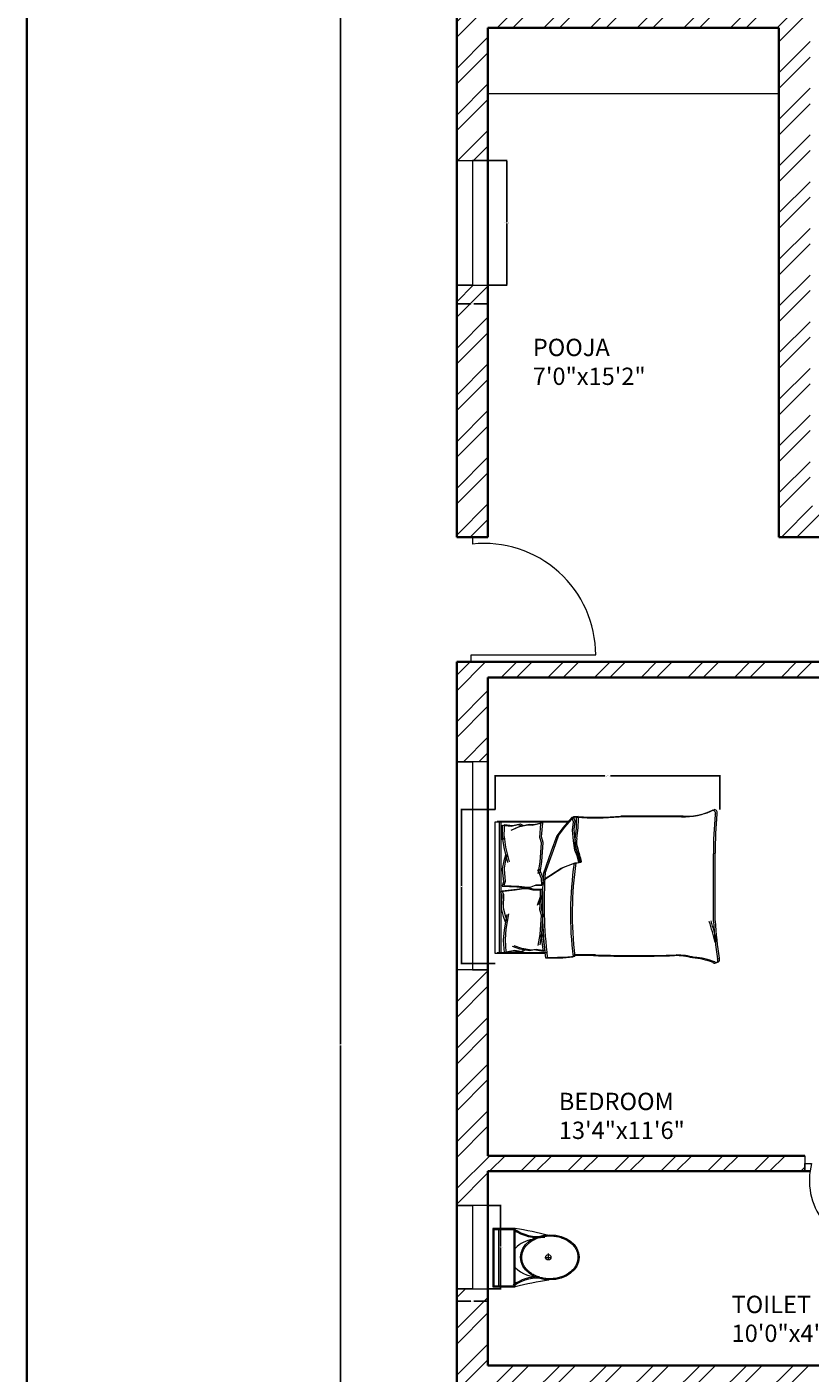
# Model space of a CAD drawing. Units: inches. Extents: x 1152 to 2588, y 1459 to 2618.
# Tile 4 of 17: x 1152 to 1378, y 1843 to 2231. Entities that reach past the tile are written whole.
import ezdxf

# ---------------------------------------------------------------- set-up
doc = ezdxf.new("R2010")
doc.units = ezdxf.units.IN
for name, color, linetype, lineweight in [('A-ANNO-DIMS', 2, 'Continuous', 18), ('A-ANNO-TTLB', 7, 'Continuous', 35), ('A-AREA-IDEN', 7, 'Continuous', 18), ('A-DOOR', 4, 'Continuous', 18), ('A-FLOR-CASE', 30, 'Continuous', 18), ('A-FLOR-FIXT', 9, 'Continuous', 18), ('A-FURN', 8, 'Continuous', 13), ('A-GLAZ', 4, 'Continuous', 18), ('A-WALL', 7, 'Continuous', 35), ('A-WALL-PATT', 8, 'Continuous', 13)]:
    doc.layers.add(name, color=color, linetype=linetype, lineweight=lineweight)
doc.styles.get("Standard").update_dxf_attribs({"font": 'arial.ttf'})
doc.dimstyles.get("Standard").update_dxf_attribs({"dimtxt": 0.18, "dimasz": 0.18, "dimexe": 0.18, "dimexo": 0.0625, "dimgap": 0.09, "dimtad": 0, "dimtih": 1, "dimtoh": 1, "dimdec": 4, "dimzin": 0, "dimdsep": 46, "dimtxsty": 'Standard', "dimcen": 0.09, "dimadec": 0, "dimazin": 0, "dimtfac": 1, "dimtdec": 4, "dimtofl": 0, "dimtmove": 0, "dimatfit": 3, "dimfxl": 1, "dimtolj": 1, "dimtzin": 0, "dimarcsym": 0})

# ---------------------------------------------------------------- blocks, each defined once
blk = doc.blocks.new('A$C31115884')
for p, q in [((283, 498), (223, 498)), ((258, 466), (258, 523)), ((0, 200), (0, 0)), ((520, 200), (0, 200)), ((10, 190), (10, 10)), ((510, 190), (10, 190)), ((510, 10), (510, 190)), ((520, 0), (520, 200)), ((510, 54), (0, 54)), ((10, 10), (510, 10)), ((0, 0), (520, 0))]:
    blk.add_line(p, q)
blk.add_circle((256, 496), 23.6)
for centre, radius, start, end in [((2778, -205), 2807, 165.4549, 171.7133), ((3237, 905), 2807, 188.2867, 194.5451), ((-295, 403), 365, 324.2091, 9.3499), ((-295, 403), 375, 324.2091, 9.3499), ((139, 406), 293, 315.8436, 2.6563), ((806, 403), 375, 179.2036, 215.7909), ((806, 403), 365, 170.6501, 215.7909), ((384, 406), 293, 190.2774, 224.1564)]:
    blk.add_arc(centre, radius, start, end)
blk.add_ellipse((256, 510), major_axis=(0, -261), ratio=0.772727)
blk.add_open_spline([(256, 259), (263, 259), (270, 260), (288, 262), (299, 265), (320, 273), (330, 278), (350, 291), (360, 299), (378, 316), (386, 326), (402, 347), (409, 358), (421, 383), (427, 395), (436, 422), (440, 436), (445, 465), (447, 480), (448, 509), (448, 524), (445, 553), (443, 568), (436, 596), (432, 610), (422, 636), (416, 649), (402, 672), (395, 683), (379, 703), (370, 712), (351, 728), (341, 735), (321, 746), (310, 751), (289, 757), (278, 759), (256, 761), (245, 761), (223, 757), (212, 754), (191, 746), (181, 741), (161, 728), (151, 720), (133, 703), (125, 693), (110, 672), (103, 660), (90, 636), (85, 623), (76, 596), (72, 582), (67, 553), (66, 538), (64, 509), (65, 494), (68, 465), (70, 450), (77, 422), (81, 408), (91, 382), (97, 370), (111, 346), (118, 335), (135, 316), (144, 307), (162, 291), (172, 284), (193, 273), (203, 269), (225, 262), (236, 260), (250, 259), (253, 259), (256, 259)], degree=3, knots=[0, 0, 0, 0, 0.110105, 0.110105, 0.285049, 0.285049, 0.459994, 0.459994, 0.634938, 0.634938, 0.809882, 0.809882, 0.984827, 0.984827, 1.159771, 1.159771, 1.334715, 1.334715, 1.50966, 1.50966, 1.684604, 1.684604, 1.859549, 1.859549, 2.034493, 2.034493, 2.209437, 2.209437, 2.384382, 2.384382, 2.559326, 2.559326, 2.73427, 2.73427, 2.909215, 2.909215, 3.084159, 3.084159, 3.259103, 3.259103, 3.434048, 3.434048, 3.608992, 3.608992, 3.783936, 3.783936, 3.958881, 3.958881, 4.133825, 4.133825, 4.30877, 4.30877, 4.483714, 4.483714, 4.658658, 4.658658, 4.833603, 4.833603, 5.008547, 5.008547, 5.183491, 5.183491, 5.358436, 5.358436, 5.53338, 5.53338, 5.708324, 5.708324, 5.883269, 5.883269, 6.058213, 6.058213, 6.233158, 6.233158, 6.283185, 6.283185, 6.283185, 6.283185])
blk = doc.blocks.new('BED-PLAN')
for p, q in [((49.83, 41.36), (64.23, 41.36)), ((49.83, 41.36), (64.23, 41.36)), ((50.34, 41.54), (64.74, 41.54)), ((50.34, 41.54), (64.74, 41.54)), ((51.02, 36.75), (50.45, 40.8)), ((50.45, 40.8), (52.97, 40.34)), ((51.02, 36.75), (50.45, 40.8)), ((50.45, 40.8), (52.97, 40.34)), ((51.53, 36.93), (50.95, 40.98)), ((50.95, 40.98), (53.48, 40.52)), ((51.53, 36.93), (50.95, 40.98)), ((50.95, 40.98), (53.48, 40.52)), ((51.81, 39.05), (51.28, 35.85)), ((51.81, 39.05), (51.28, 35.85)), ((52.32, 39.23), (51.79, 36.03)), ((52.32, 39.23), (51.79, 36.03)), ((52.97, 40.34), (54.24, 40.57)), ((52.97, 40.34), (54.24, 40.57)), ((53.48, 40.52), (54.75, 40.75)), ((53.48, 40.52), (54.75, 40.75)), ((54.24, 40.57), (57.11, 40.11)), ((54.24, 40.57), (57.11, 40.11)), ((54.75, 40.75), (57.62, 40.29)), ((54.75, 40.75), (57.62, 40.29)), ((57, 40.91), (56.19, 40.45)), ((57, 40.91), (56.19, 40.45)), ((57.51, 41.09), (56.7, 40.64)), ((57.51, 41.09), (56.7, 40.64)), ((59.07, 40.57), (57, 40.91)), ((59.07, 40.57), (57, 40.91)), ((57.11, 40.11), (59.3, 39.3)), ((57.11, 40.11), (59.3, 39.3)), ((59.57, 40.75), (57.51, 41.09)), ((59.57, 40.75), (57.51, 41.09)), ((57.62, 40.29), (59.8, 39.49)), ((57.62, 40.29), (59.8, 39.49)), ((61.59, 41.03), (59.07, 40.57)), ((61.59, 41.03), (59.07, 40.57)), ((62.1, 41.21), (59.57, 40.75)), ((62.1, 41.21), (59.57, 40.75)), ((61.58, 41.03), (61.84, 37.62)), ((61.58, 41.02), (61.84, 37.62)), ((62.08, 41.21), (62.35, 37.8)), ((62.08, 41.21), (62.35, 37.8)), ((63.01, 41.36), (63.01, 3.37)), ((63.01, 41.36), (63.01, 3.37)), ((63.52, 41.54), (63.52, 3.56)), ((63.52, 41.54), (63.52, 3.56)), ((64.74, 41.54), (64.74, 3.56)), ((51.28, 35.85), (50.93, 30.27)), ((51.28, 35.85), (50.93, 30.27)), ((51.28, 35.85), (51.02, 36.75)), ((51.28, 35.85), (51.02, 36.75)), ((51.79, 36.03), (51.44, 30.46)), ((51.79, 36.03), (51.44, 30.46)), ((51.79, 36.03), (51.53, 36.93)), ((51.79, 36.03), (51.53, 36.93)), ((61.82, 37.54), (61.59, 34.5)), ((61.82, 37.54), (61.59, 34.5)), ((61.84, 37.62), (61.82, 37.54)), ((61.84, 37.62), (61.82, 37.54)), ((62.33, 37.72), (62.1, 34.68)), ((62.33, 37.72), (62.1, 34.68)), ((62.35, 37.8), (62.33, 37.72)), ((62.35, 37.8), (62.33, 37.72)), ((1.24, 32.15), (1.24, 12.59)), ((1.24, 32.15), (1.24, 12.59)), ((1.75, 32.33), (1.75, 12.77)), ((1.75, 32.33), (1.75, 12.77)), ((61.59, 34.5), (60.79, 30.13)), ((61.59, 34.5), (60.79, 30.13)), ((61.25, 32.32), (61.82, 30.71)), ((61.25, 32.32), (61.82, 30.71)), ((62.1, 34.68), (61.3, 30.31)), ((62.1, 34.68), (61.3, 30.31)), ((61.76, 32.5), (62.33, 30.89)), ((61.76, 32.5), (62.33, 30.89)), ((50.93, 30.27), (51.38, 28.72)), ((50.93, 30.27), (51.38, 28.72)), ((51.38, 28.72), (51.06, 24.64)), ((51.38, 28.72), (51.06, 24.64)), ((51.3, 24.96), (52.17, 27.46)), ((51.3, 24.96), (52.17, 27.46)), ((51.44, 30.46), (51.89, 28.9)), ((51.44, 30.46), (51.89, 28.9)), ((51.89, 28.9), (51.56, 24.82)), ((51.89, 28.9), (51.56, 24.82)), ((51.81, 25.15), (52.68, 27.65)), ((51.81, 25.15), (52.68, 27.65)), ((61.82, 30.71), (62.4, 28.41)), ((61.82, 30.71), (62.4, 28.41)), ((62.4, 28.15), (62.28, 24.62)), ((62.4, 28.15), (62.28, 24.62)), ((62.33, 30.89), (62.91, 28.59)), ((62.33, 30.89), (62.91, 28.59)), ((62.4, 28.41), (62.4, 28.15)), ((62.4, 28.41), (62.4, 28.15)), ((62.91, 28.34), (62.79, 24.8)), ((62.91, 28.34), (62.79, 24.8)), ((62.91, 28.59), (62.91, 28.34)), ((62.91, 28.59), (62.91, 28.34)), ((51.3, 23.01), (51.3, 24.96)), ((51.3, 23.01), (51.3, 24.96)), ((51.81, 23.19), (51.81, 25.15)), ((51.81, 23.19), (51.81, 25.15)), ((62.74, 23.47), (58.49, 23.01)), ((62.74, 23.47), (58.49, 23.01)), ((63.25, 23.65), (59, 23.19)), ((63.25, 23.65), (59, 23.19)), ((62.28, 24.62), (62.74, 23.47)), ((62.28, 24.62), (62.74, 23.47)), ((62.79, 24.8), (63.25, 23.65)), ((62.79, 24.8), (63.25, 23.65)), ((50.41, 20.07), (45.25, 16.74)), ((50.41, 20.07), (45.25, 16.74)), ((50.92, 20.25), (45.76, 16.92)), ((50.92, 20.25), (45.76, 16.92)), ((52.93, 21.76), (50.8, 21.63)), ((52.93, 21.76), (50.8, 21.63)), ((50.8, 21.63), (50.92, 19.68)), ((50.8, 21.63), (50.92, 19.68)), ((50.92, 19.68), (51.95, 17.24)), ((50.92, 19.68), (51.95, 17.24)), ((53.43, 23.01), (51.3, 23.01)), ((53.43, 23.01), (51.3, 23.01)), ((53.44, 21.95), (51.31, 21.81)), ((53.44, 21.94), (51.31, 21.81)), ((51.31, 21.81), (51.43, 19.86)), ((51.31, 21.81), (51.43, 19.86)), ((51.43, 19.86), (52.45, 17.42)), ((51.43, 19.86), (52.45, 17.42)), ((53.94, 23.19), (51.81, 23.19)), ((53.94, 23.19), (51.81, 23.19)), ((54.39, 22.32), (52.93, 21.76)), ((54.39, 22.32), (52.93, 21.76)), ((54.93, 22.55), (53.43, 23.01)), ((54.93, 22.55), (53.43, 23.01)), ((54.9, 22.5), (53.44, 21.94)), ((54.9, 22.5), (53.44, 21.95)), ((55.44, 22.73), (53.94, 23.19)), ((55.44, 22.73), (53.94, 23.19)), ((55.42, 22.38), (54.39, 22.32)), ((55.42, 22.38), (54.39, 22.32)), ((55.93, 22.56), (54.9, 22.5)), ((55.93, 22.56), (54.9, 22.5)), ((55.96, 22.55), (54.93, 22.55)), ((55.96, 22.55), (54.93, 22.55)), ((57.98, 22.08), (55.42, 22.38)), ((57.98, 22.08), (55.42, 22.38)), ((56.47, 22.73), (55.44, 22.73)), ((56.47, 22.73), (55.44, 22.73)), ((58.48, 22.26), (55.93, 22.56)), ((58.48, 22.26), (55.93, 22.56)), ((58.49, 23.01), (55.96, 22.55)), ((58.49, 23.01), (55.96, 22.55)), ((59, 23.19), (56.47, 22.73)), ((59, 23.19), (56.47, 22.73)), ((62.25, 21.89), (57.98, 22.08)), ((62.25, 21.89), (57.98, 22.08)), ((62.76, 22.07), (58.48, 22.26)), ((62.76, 22.07), (58.48, 22.26)), ((61.86, 20.71), (62.25, 21.89)), ((61.86, 20.71), (62.25, 21.89)), ((62.2, 17.19), (61.86, 20.71)), ((62.2, 17.19), (61.86, 20.71)), ((62.37, 20.89), (62.76, 22.07)), ((62.37, 20.89), (62.76, 22.07)), ((62.71, 17.37), (62.37, 20.89)), ((62.71, 17.37), (62.37, 20.89)), ((42.19, 15.57), (40.59, 15.32)), ((42.19, 15.57), (40.59, 15.32)), ((45.25, 16.74), (41.68, 15.39)), ((45.25, 16.74), (41.68, 15.39)), ((45.76, 16.92), (42.19, 15.57)), ((45.76, 16.92), (42.19, 15.57)), ((48.08, 11.82), (50.41, 18.44)), ((48.08, 11.82), (50.41, 18.44)), ((48.59, 12), (50.92, 18.63)), ((48.59, 12), (50.92, 18.63)), ((51.81, 18.24), (51.28, 15.03)), ((51.81, 18.24), (51.28, 15.03)), ((52.32, 18.42), (51.79, 15.22)), ((52.32, 18.42), (51.79, 15.22)), ((61.78, 14.61), (62.21, 16.94)), ((61.78, 14.61), (62.21, 16.94)), ((62.21, 16.94), (62.2, 17.19)), ((62.21, 16.94), (62.2, 17.19)), ((62.29, 14.79), (62.72, 17.12)), ((62.29, 14.79), (62.72, 17.12)), ((62.72, 17.12), (62.71, 17.37)), ((62.72, 17.12), (62.71, 17.37)), ((41.68, 15.39), (40.08, 15.14)), ((41.68, 15.39), (40.08, 15.14)), ((40.08, 15.14), (40.58, 13.17)), ((40.08, 15.14), (40.58, 13.17)), ((40.58, 13.17), (41.31, 11.57)), ((40.58, 13.17), (41.31, 11.57)), ((40.59, 15.32), (41.08, 13.35)), ((40.59, 15.32), (41.08, 13.35)), ((41.08, 13.35), (41.82, 11.75)), ((41.08, 13.35), (41.82, 11.75)), ((41.82, 11.75), (42.19, 9.04)), ((41.82, 11.75), (42.19, 9.04)), ((46.48, 7.38), (48.08, 11.82)), ((46.48, 7.38), (48.08, 11.82)), ((46.99, 7.57), (48.59, 12)), ((46.99, 7.57), (48.59, 12)), ((51.28, 15.03), (50.93, 9.46)), ((51.28, 15.03), (50.93, 9.46)), ((51.79, 15.22), (51.44, 9.64)), ((51.79, 15.22), (51.44, 9.64)), ((61.79, 10.81), (60.71, 15.11)), ((61.79, 10.81), (60.71, 15.11)), ((62.3, 10.99), (61.22, 15.3)), ((62.3, 10.99), (61.22, 15.3)), ((61.31, 12.96), (61.78, 14.61)), ((61.31, 12.96), (61.78, 14.61)), ((61.82, 13.15), (62.29, 14.79)), ((61.82, 13.15), (62.29, 14.79)), ((41.31, 11.57), (41.68, 8.86)), ((41.31, 11.57), (41.68, 8.86)), ((41.68, 8.86), (41.93, 5.78)), ((41.68, 8.86), (41.93, 5.78)), ((42.19, 9.04), (42.44, 5.97)), ((42.19, 9.04), (42.44, 5.97)), ((50.93, 9.46), (51.38, 7.9)), ((50.93, 9.46), (51.38, 7.9)), ((51.38, 7.9), (51.06, 3.82)), ((51.38, 7.9), (51.06, 3.82)), ((51.44, 9.64), (51.89, 8.09)), ((51.44, 9.64), (51.89, 8.09)), ((51.89, 8.09), (51.56, 4.01)), ((51.89, 8.09), (51.56, 4.01)), ((62.21, 7.79), (61.79, 10.81)), ((62.21, 7.79), (61.79, 10.81)), ((62.2, 4.29), (62.27, 8.59)), ((62.2, 4.29), (62.27, 8.58)), ((62.27, 8.59), (62.21, 7.79)), ((62.27, 8.58), (62.21, 7.79)), ((62.72, 7.97), (62.3, 10.99)), ((62.72, 7.97), (62.3, 10.99)), ((62.71, 4.47), (62.78, 8.77)), ((62.71, 4.47), (62.78, 8.77)), ((62.78, 8.77), (62.72, 7.97)), ((62.78, 8.77), (62.72, 7.97)), ((41.93, 5.78), (41.68, 3.32)), ((41.93, 5.78), (41.68, 3.32)), ((42.18, 2.1), (44.76, 5.05)), ((42.18, 2.1), (44.76, 5.05)), ((42.44, 5.97), (42.19, 3.5)), ((42.44, 5.97), (42.19, 3.5)), ((42.68, 2.28), (45.27, 5.23)), ((42.68, 2.28), (45.27, 5.23)), ((44.76, 5.05), (46.48, 7.38)), ((44.76, 5.05), (46.48, 7.38)), ((45.27, 5.23), (46.99, 7.57)), ((45.27, 5.23), (46.99, 7.57)), ((51.06, 3.82), (53.55, 4.44)), ((51.06, 3.82), (53.55, 4.44)), ((51.56, 4.01), (54.06, 4.62)), ((51.56, 4.01), (54.06, 4.62)), ((53.55, 4.44), (54.83, 4.29)), ((53.55, 4.44), (54.83, 4.29)), ((54.06, 4.62), (55.34, 4.47)), ((54.06, 4.62), (55.34, 4.47)), ((54.83, 4.29), (57.67, 4.93)), ((54.83, 4.29), (57.67, 4.93)), ((55.34, 4.47), (58.17, 5.11)), ((55.34, 4.47), (58.17, 5.11)), ((57.6, 4.12), (56.77, 4.53)), ((57.6, 4.12), (56.77, 4.53)), ((58.11, 4.3), (57.28, 4.71)), ((58.11, 4.3), (57.28, 4.71)), ((59.65, 4.59), (57.6, 4.12)), ((59.65, 4.59), (57.6, 4.12)), ((57.67, 4.93), (59.8, 5.87)), ((57.67, 4.93), (59.8, 5.87)), ((60.15, 4.77), (58.11, 4.3)), ((60.15, 4.77), (58.11, 4.3)), ((58.17, 5.11), (60.3, 6.05)), ((58.17, 5.11), (60.3, 6.05)), ((62.2, 4.29), (59.65, 4.59)), ((62.2, 4.29), (59.65, 4.59)), ((62.71, 4.47), (60.15, 4.77)), ((62.71, 4.47), (60.15, 4.77)), ((40.79, 2.04), (42.18, 2.1, 3.08)), ((40.79, 2.04), (42.18, 2.1, 3.08)), ((41.3, 2.22), (42.68, 2.28, 3.08)), ((41.3, 2.22), (42.68, 2.28, 3.08)), ((41.68, 3.32), (42.18, 2.1)), ((41.68, 3.32), (42.18, 2.1)), ((42.19, 3.5), (42.68, 2.28)), ((42.19, 3.5), (42.68, 2.28)), ((64.23, 3.37), (43.08, 3.37)), ((64.23, 3.37), (43.08, 3.37)), ((64.74, 3.56), (43.59, 3.56)), ((64.74, 3.56), (43.59, 3.56))]:
    blk.add_line(p, q)
for centre, radius, start, end in [((0.86, 43.26), 0.866, 56.1736, 203.4781), ((0.86, 43.26), 0.866, 56.1736, 203.4781), ((-95.41, 27.09), 96.78, 2.9958, 9.4091), ((-95.41, 27.09), 96.78, 2.9958, 9.4091), ((1.37, 43.44), 0.866, 56.1736, 203.4781), ((1.37, 43.44), 0.866, 56.1736, 203.4781), ((-94.9, 27.27), 96.78, 2.9958, 9.4091), ((-94.9, 27.27), 96.78, 2.9958, 9.4091), ((8.37, 61.34), 18.73, 247.9751, 266.652), ((8.37, 61.34), 18.73, 247.9751, 266.652), ((8.88, 61.52), 18.73, 247.9751, 266.652), ((8.88, 61.52), 18.73, 247.9751, 266.652), ((13.46, 65.69), 23.56, 256.0648, 268.9113), ((13.46, 65.69), 23.56, 256.0648, 268.9113), ((48.76, -23.39), 66.22, 88.7218, 95.604), ((48.76, -23.39), 66.22, 88.7218, 95.604), ((-79.97, 27.33), 131.13, 356.0865, 6.7821), ((-79.97, 27.33), 131.13, 356.0865, 6.7821), ((12.95, 65.51), 23.56, 256.0648, 268.9113), ((12.95, 65.51), 23.56, 256.0648, 268.9113), ((24, -341.25), 383.38, 88.2277, 91.7185), ((24, -341.25), 383.38, 88.2277, 91.7185), ((24.51, -341.07), 383.38, 88.2277, 91.7185), ((24.51, -341.07), 383.38, 88.2277, 91.7185), ((39.45, 177.11), 135.22, 268.4762, 271.0082), ((39.45, 177.11), 135.22, 268.4762, 271.0082), ((39.96, 177.3), 135.22, 268.4762, 271.0082), ((39.96, 177.3), 135.22, 268.4762, 271.0082), ((-60.02, 30.01), 102.56, 351.7845, 6.9006), ((-60.02, 30.01), 102.56, 351.7845, 6.9006), ((48.26, -23.57), 66.22, 88.7218, 95.604), ((48.26, -23.57), 66.22, 88.7218, 95.604), ((-59.52, 30.19), 102.56, 351.7845, 6.9006), ((-59.52, 30.19), 102.56, 351.7845, 6.9006), ((-80.48, 27.15), 131.13, 356.0865, 6.7821), ((-80.48, 27.15), 131.13, 356.0865, 6.7821), ((83.08, 57.81), 84.62, 193.3832, 197.7053), ((83.08, 57.81), 84.62, 193.3832, 197.7053), ((83.59, 57.99), 84.62, 193.3832, 197.7053), ((83.59, 57.99), 84.62, 193.3832, 197.7053), ((-104.51, 11.41), 105.75, 354.4998, 0.6351), ((-104.51, 11.41), 105.75, 354.4998, 0.6351), ((-104, 11.59), 105.75, 354.4998, 0.6351), ((-104, 11.59), 105.75, 354.4998, 0.6351), ((40.03, 15), 0.147, 70.2464, 181.1377), ((40.03, 15), 0.147, 70.2464, 181.1377), ((63.05, 19.36), 23.57, 190.6617, 199.8806), ((63.05, 19.36), 23.57, 190.6617, 199.8806), ((40.54, 15.18), 0.147, 70.2464, 181.1377), ((40.54, 15.18), 0.147, 70.2464, 181.1377), ((63.56, 19.54), 23.57, 190.6617, 199.8806), ((63.56, 19.54), 23.57, 190.6617, 199.8806), ((69.52, 3.32), 28.76, 169.8763, 182.5657), ((69.52, 3.32), 28.76, 169.8763, 182.5657), ((36.36, 9.35), 4.95, 348.6608, 23.7384), ((36.36, 9.35), 4.95, 348.6608, 23.7384), ((70.03, 3.51), 28.76, 169.8763, 182.5657), ((70.03, 3.51), 28.76, 169.8763, 182.5657), ((36.86, 9.53), 4.95, 348.6608, 23.7384), ((36.86, 9.53), 4.95, 348.6608, 23.7384), ((1.54, 0.87), 0.876, 152.6588, 266.02), ((1.54, 0.87), 0.876, 152.6588, 266.02), ((2.05, 1.06), 0.876, 152.6588, 266.02), ((2.05, 1.06), 0.876, 152.6588, 266.02), ((9.65, -16.41), 18.33, 87.4714, 116.4681), ((9.65, -16.41), 18.33, 87.4714, 116.4681), ((10.16, -16.23), 18.33, 87.4714, 116.4681), ((10.16, -16.23), 18.33, 87.4714, 116.4681), ((10.32, 3628.06), 3626.16, 270.00217, 270.28689), ((10.32, 3628.06), 3626.16, 270.00217, 270.28689), ((10.83, 3628.24), 3626.16, 270.00217, 270.28689), ((10.83, 3628.24), 3626.16, 270.00217, 270.28689), ((35.36, -100.76), 102.94, 86.9791, 93.8365), ((35.36, -100.76), 102.94, 86.9791, 93.8365), ((35.87, -100.58), 102.94, 86.9791, 93.8365), ((35.87, -100.57), 102.94, 86.9791, 93.8365)]:
    blk.add_arc(centre, radius, start, end)
blk = doc.blocks.new('DOOR-24-BATH-WEST')
for p, q in [((0, 26.25), (0, 21.75)), ((0, 21.75), (0, 24)), ((0, 24), (2, 24)), ((22.43, 24), (20.43, 24)), ((20.43, 24), (20.43, 0)), ((22.43, 21.75), (22.43, 26.25)), ((22.43, 26.25), (22.43, 24))]:
    blk.add_line(p, q)
blk.add_arc((20.43, 19.08), 19.08, 165.0504, 270)
blk = doc.blocks.new('DOOR-36-POOJA')
for p, q in [((0.4, 36), (0.4, 34)), ((0, 0), (0, 2)), ((0, 2), (36, 2))]:
    blk.add_line(p, q)
blk.add_arc((3.82, 2), 32.18, 0, 96.1017)
blk = doc.blocks.new('WIN-60-EXT')
for p, q in [((0, 9), (0, 0)), ((60, 4.5), (60, 9)), ((60, 9), (60, 0)), ((0, 0), (0, 4.5)), ((0, 4.5), (60, 4.5))]:
    blk.add_line(p, q)
blk = doc.blocks.new('WIN-36')
for p, q in [((0, 36), (9, 36)), ((9, 36), (4.5, 36)), ((4.5, 36), (4.5, 0)), ((4.5, 0), (0, 0)), ((0, 0), (9, 0))]:
    blk.add_line(p, q)
blk = doc.blocks.new('WIN-24-BATH-WEST')
for p, q in [((9, 24), (0, 24)), ((0, 24), (4.5, 24)), ((4.5, 24), (4.5, 0)), ((4.5, 0), (0, 0)), ((0, 0), (9, 0))]:
    blk.add_line(p, q)
blk = doc.blocks.new('*D28')
at = {"layer": 'A-ANNO-DIMS', "color": 0, "lineweight": -2, "transparency": 16777216}
for p, q in [((1285.48, 2192.75), (1291, 2192.75)), ((1290.82, 2192.57), (1290.82, 2174.93)), ((1290.82, 2156.93), (1290.82, 2174.57)), ((1285.48, 2156.75), (1291, 2156.75))]:
    blk.add_line(p, q, dxfattribs=at)
at = {"layer": 'A-ANNO-DIMS', "color": 0, "transparency": 16777216}
for points in [[(1290.79, 2192.57), (1290.85, 2192.57), (1290.82, 2192.75)], [(1290.79, 2156.93), (1290.85, 2156.93), (1290.82, 2156.75)]]:
    blk.add_solid(points, dxfattribs=at)
at = {"layer": 'Defpoints', "color": 0, "transparency": 16777216}
for p in [(1285.42, 2192.75), (1290.82, 2192.75), (1285.42, 2156.75)]:
    blk.add_point(p, dxfattribs=at)
at = {"layer": 'A-ANNO-DIMS', "color": 0, "transparency": 16777216, "insert": (1290.82, 2174.75), "char_height": 0.18, "attachment_point": 5}
blk.add_mtext('\\A1;WIN. 36 TYP.', dxfattribs=at)
blk = doc.blocks.new('*D29')
at = {"layer": 'A-ANNO-DIMS', "color": 0, "lineweight": -2, "transparency": 16777216}
for p, q in [((1276.42, 2156.69), (1276.42, 2151.17)), ((1285.42, 2156.69), (1285.42, 2151.17)), ((1276.6, 2151.35), (1280.46, 2151.35)), ((1285.24, 2151.35), (1281.37, 2151.35))]:
    blk.add_line(p, q, dxfattribs=at)
at = {"layer": 'A-ANNO-DIMS', "color": 0, "transparency": 16777216}
for points in [[(1276.6, 2151.38), (1276.6, 2151.32), (1276.42, 2151.35)], [(1285.24, 2151.38), (1285.24, 2151.32), (1285.42, 2151.35)]]:
    blk.add_solid(points, dxfattribs=at)
at = {"layer": 'Defpoints', "color": 0, "transparency": 16777216}
for p in [(1276.42, 2156.75), (1285.42, 2156.75), (1285.42, 2151.35)]:
    blk.add_point(p, dxfattribs=at)
at = {"layer": 'A-ANNO-DIMS', "color": 0, "transparency": 16777216, "insert": (1280.92, 2151.35), "char_height": 0.18, "attachment_point": 5}
blk.add_mtext('\\A1;9 TYP.', dxfattribs=at)
blk = doc.blocks.new('*D32')
at = {"layer": 'A-ANNO-DIMS', "color": 0, "lineweight": -2, "transparency": 16777216}
for p, q in [((1287.53, 2005.5), (1287.53, 2015.34)), ((1287.71, 2015.16), (1319.13, 2015.16)), ((1352.17, 2015.16), (1320.76, 2015.16)), ((1352.35, 2005.5), (1352.35, 2015.34))]:
    blk.add_line(p, q, dxfattribs=at)
at = {"layer": 'A-ANNO-DIMS', "color": 0, "transparency": 16777216}
for points in [[(1287.71, 2015.19), (1287.71, 2015.13), (1287.53, 2015.16)], [(1352.17, 2015.19), (1352.17, 2015.13), (1352.35, 2015.16)]]:
    blk.add_solid(points, dxfattribs=at)
at = {"layer": 'Defpoints', "color": 0, "transparency": 16777216}
for p in [(1287.53, 2015.16), (1287.53, 2005.43), (1352.35, 2005.43)]:
    blk.add_point(p, dxfattribs=at)
at = {"layer": 'A-ANNO-DIMS', "color": 0, "transparency": 16777216, "insert": (1319.94, 2015.16), "char_height": 0.18, "attachment_point": 5}
blk.add_mtext('\\A1;BED 65 TYP.', dxfattribs=at)
blk = doc.blocks.new('*D33')
at = {"layer": 'A-ANNO-DIMS', "color": 0, "lineweight": -2, "transparency": 16777216}
for p, q in [((1287.47, 2005.43), (1277.63, 2005.43)), ((1277.81, 2005.25), (1277.81, 1983.43)), ((1277.81, 1961.24), (1277.81, 1983.07)), ((1287.47, 1961.06), (1277.63, 1961.06))]:
    blk.add_line(p, q, dxfattribs=at)
at = {"layer": 'A-ANNO-DIMS', "color": 0, "transparency": 16777216}
for points in [[(1277.78, 2005.25), (1277.84, 2005.25), (1277.81, 2005.43)], [(1277.78, 1961.24), (1277.84, 1961.24), (1277.81, 1961.06)]]:
    blk.add_solid(points, dxfattribs=at)
at = {"layer": 'Defpoints', "color": 0, "transparency": 16777216}
for p in [(1287.53, 2005.43), (1277.81, 1961.06), (1287.53, 1961.06)]:
    blk.add_point(p, dxfattribs=at)
at = {"layer": 'A-ANNO-DIMS', "color": 0, "transparency": 16777216, "insert": (1277.81, 1983.25), "char_height": 0.18, "attachment_point": 5}
blk.add_mtext('\\A1;44 TYP.', dxfattribs=at)
blk = doc.blocks.new('*D56')
at = {"layer": 'A-ANNO-DIMS', "color": 0, "lineweight": -2, "transparency": 16777216}
for p, q in [((1285.48, 1891.13), (1289.2, 1891.13)), ((1289.02, 1890.95), (1289.02, 1879.31)), ((1289.02, 1867.31), (1289.02, 1878.95)), ((1285.48, 1867.13), (1289.2, 1867.13))]:
    blk.add_line(p, q, dxfattribs=at)
at = {"layer": 'A-ANNO-DIMS', "color": 0, "transparency": 16777216}
for points in [[(1288.99, 1890.95), (1289.05, 1890.95), (1289.02, 1891.13)], [(1288.99, 1867.31), (1289.05, 1867.31), (1289.02, 1867.13)]]:
    blk.add_solid(points, dxfattribs=at)
at = {"layer": 'Defpoints', "color": 0, "transparency": 16777216}
for p in [(1285.42, 1891.13), (1289.02, 1891.13), (1285.42, 1867.13)]:
    blk.add_point(p, dxfattribs=at)
at = {"layer": 'A-ANNO-DIMS', "color": 0, "transparency": 16777216, "insert": (1289.02, 1879.13), "char_height": 0.18, "attachment_point": 5}
blk.add_mtext('\\A1;WIN. 24 TYP.', dxfattribs=at)
blk = doc.blocks.new('*D57')
at = {"layer": 'A-ANNO-DIMS', "color": 0, "lineweight": -2, "transparency": 16777216}
for p, q in [((1276.42, 1867.07), (1276.42, 1863.35)), ((1285.42, 1867.07), (1285.42, 1863.35)), ((1276.6, 1863.53), (1280.46, 1863.53)), ((1285.24, 1863.53), (1281.37, 1863.53))]:
    blk.add_line(p, q, dxfattribs=at)
at = {"layer": 'A-ANNO-DIMS', "color": 0, "transparency": 16777216}
for points in [[(1276.6, 1863.56), (1276.6, 1863.5), (1276.42, 1863.53)], [(1285.24, 1863.56), (1285.24, 1863.5), (1285.42, 1863.53)]]:
    blk.add_solid(points, dxfattribs=at)
at = {"layer": 'Defpoints', "color": 0, "transparency": 16777216}
for p in [(1276.42, 1867.13), (1285.42, 1867.13), (1285.42, 1863.53)]:
    blk.add_point(p, dxfattribs=at)
at = {"layer": 'A-ANNO-DIMS', "color": 0, "transparency": 16777216, "insert": (1280.92, 1863.53), "char_height": 0.18, "attachment_point": 5}
blk.add_mtext('\\A1;9 TYP.', dxfattribs=at)
blk = doc.blocks.new('*D71')
at = {"layer": 'A-ANNO-DIMS', "color": 0, "lineweight": -2, "transparency": 16777216}
for p, q in [((1276.35, 2240.05), (1242.64, 2240.05)), ((1242.82, 2239.87), (1242.82, 1937.73)), ((1242.82, 1635.23), (1242.82, 1937.36)), ((1276.35, 1635.05), (1242.64, 1635.05))]:
    blk.add_line(p, q, dxfattribs=at)
at = {"layer": 'A-ANNO-DIMS', "color": 0, "transparency": 16777216}
for points in [[(1242.79, 2239.87), (1242.85, 2239.87), (1242.82, 2240.05)], [(1242.79, 1635.23), (1242.85, 1635.23), (1242.82, 1635.05)]]:
    blk.add_solid(points, dxfattribs=at)
at = {"layer": 'Defpoints', "color": 0, "transparency": 16777216}
for p in [(1242.82, 2240.05), (1276.42, 2240.05), (1276.42, 1635.05)]:
    blk.add_point(p, dxfattribs=at)
at = {"layer": 'A-ANNO-DIMS', "color": 0, "transparency": 16777216, "insert": (1242.82, 1937.55), "char_height": 0.18, "attachment_point": 5}
blk.add_mtext('\\A1;605', dxfattribs=at)

msp = doc.modelspace()

# ---------------------------------------------------------------- hatches: boundary and pattern name
at = {"layer": 'A-WALL-PATT'}
h = msp.add_hatch(dxfattribs=at)
h.set_pattern_fill('ANSI32', color=256)
h.paths.add_polyline_path([(1408.9272, 2240.0458), (1276.4165, 2240.0458), (1276.4165, 2192.7491), (1285.4165, 2192.7491), (1285.4165, 2231.0458), (1369.4165, 2231.0458), (1369.4165, 2084.0458), (1526.9165, 2084.0458), (1526.9165, 2096.3728), (1524.6665, 2096.3728), (1522.4165, 2096.3728), (1522.4165, 2093.0458), (1378.4165, 2093.0458), (1378.4165, 2231.0458), (1408.9272, 2231.0458)])
h.paths.add_polyline_path([(1736.4165, 2240.0458), (1468.9272, 2240.0458), (1468.9272, 2231.0458), (1522.4165, 2231.0458), (1522.4165, 2127.3313), (1526.9165, 2127.3313), (1526.9165, 2231.0458), (1574.9165, 2231.0458), (1574.9165, 2188.0458), (1579.4165, 2188.0458), (1579.4165, 2231.0458), (1727.4165, 2231.0458), (1727.4165, 2183.9728), (1736.4165, 2183.9728)])
h.paths.add_polyline_path([(1285.4165, 2156.7491), (1276.4165, 2156.7491), (1276.4165, 2084.0458), (1285.4165, 2084.0458)], flags=17)
h.paths.add_polyline_path([(1285.4165, 2043.5458), (1445.4165, 2043.5458), (1445.4165, 1943.6503), (1454.4165, 1943.6503), (1454.4165, 2048.0458), (1276.4165, 2048.0458), (1276.4165, 2019.2077), (1280.9165, 2019.2077), (1285.4165, 2019.2077)])
h.paths.add_polyline_path([(1285.4165, 1959.2077), (1276.4165, 1959.2077), (1276.4165, 1891.1319), (1280.9165, 1891.1319), (1285.4165, 1891.1319), (1285.4165, 1901.0458), (1376.8505, 1901.0458), (1376.8505, 1903.2958), (1376.8505, 1905.5458), (1285.4165, 1905.5458)])
h.paths.add_polyline_path([(1518.4165, 1905.5458), (1399.2832, 1905.5458), (1399.2832, 1903.2958), (1399.2832, 1901.0458), (1405.4165, 1901.0458), (1405.4165, 1884.8579), (1409.9165, 1884.8579), (1409.9165, 1901.0458), (1513.9165, 1901.0458), (1513.9165, 1869.1706), (1518.4165, 1869.1706)])
h.paths.add_polyline_path([(1520.5229, 1845.0458), (1518.4165, 1845.0458), (1518.4165, 1849.2927), (1516.1665, 1849.2927), (1513.9165, 1849.2927), (1513.9165, 1845.0458), (1409.9165, 1845.0458), (1409.9165, 1860.8579), (1405.4165, 1860.8579), (1405.4165, 1845.0458), (1285.4165, 1845.0458), (1285.4165, 1867.1319), (1276.4165, 1867.1319), (1276.4165, 1635.0458), (1285.4165, 1635.0458), (1285.4165, 1836.0458), (1405.4165, 1836.0458), (1405.4165, 1635.0458), (1414.4165, 1635.0458), (1424.7277, 1635.0458), (1424.7277, 1639.5458), (1424.7277, 1644.0458), (1414.4165, 1644.0458), (1414.4165, 1836.0458), (1414.4165, 1840.5831), (1520.5229, 1840.5831)])
h.paths.add_polyline_path([(1579.4165, 1840.5458), (1583.4035, 1840.5458), (1583.4035, 1845.0458), (1579.4165, 1845.0458), (1570.4165, 1845.0458), (1570.4165, 1840.5831), (1570.4165, 1644.0458), (1548.2359, 1644.0458), (1548.2359, 1635.0458), (1611.2801, 1635.0458), (1611.2801, 1639.5458), (1611.2801, 1644.0458), (1579.4165, 1644.0458)])
h.paths.add_polyline_path([(1488.2359, 1644.0458), (1472.0663, 1644.0458), (1472.0663, 1635.0458), (1488.2359, 1635.0458), (1488.2359, 1639.5458)], flags=17)
h.paths.add_polyline_path([(1736.4165, 1701.1863), (1727.4165, 1701.1863), (1727.4165, 1644.0458), (1671.2801, 1644.0458), (1671.2801, 1635.0458), (1736.4165, 1635.0458)])
h.paths.add_polyline_path([(1736.4165, 2147.9728), (1727.4165, 2147.9728), (1727.4165, 2093.0458), (1579.4165, 2093.0458), (1574.9165, 2093.0458), (1574.9165, 1971.6501), (1579.4165, 1971.6501), (1579.4165, 2084.0458), (1727.4165, 2084.0458), (1727.4165, 2054.3847), (1736.4165, 2054.3847)])
h.paths.add_polyline_path([(1736.4165, 1994.3847), (1727.4165, 1994.3847), (1727.4165, 1911.3562), (1736.4165, 1911.3562)])
h.paths.add_polyline_path([(1736.4165, 1875.3562), (1727.4165, 1875.3562), (1727.4165, 1845.0458), (1617.1767, 1845.0458), (1617.1767, 1842.7958), (1617.1767, 1840.5458), (1618.9165, 1840.5458), (1618.9165, 1788.5458), (1618.9165, 1784.0458), (1627.8699, 1784.0458), (1627.8699, 1788.5458), (1623.4165, 1788.5458), (1623.4165, 1840.5458), (1727.4165, 1840.5458), (1727.4165, 1828.7619), (1736.4165, 1828.7619)])
h.paths.add_polyline_path([(1727.4165, 1938.0458), (1579.4165, 1938.0458), (1579.4165, 1942.7722), (1574.9165, 1942.7722), (1574.9165, 1929.0458), (1727.4165, 1929.0458)])

# ---------------------------------------------------------------- linework, layer by layer
at = {"layer": 'A-ANNO-TTLB'}
msp.add_lwpolyline([(1152.3215, 2617.6685), (2587.6987, 2617.6685), (2587.6987, 1459.3148), (1152.3215, 1459.3148)], close=True, dxfattribs=at)
at = {"layer": 'A-FLOR-CASE'}
msp.add_line((1285.4165, 2212.1153), (1369.4165, 2212.1153), dxfattribs=at)
at = {"layer": 'A-WALL'}
for p, q in [((1276.4165, 2240.0458), (1276.4165, 2084.0458)), ((1285.4165, 2231.0458), (1369.4165, 2231.0458)), ((1285.4165, 2231.0458), (1285.4165, 2084.0458)), ((1369.4165, 2231.0458), (1369.4165, 2084.0458)), ((1276.4165, 2084.0458), (1285.4165, 2084.0458)), ((1369.4165, 2084.0458), (1526.9165, 2084.0458)), ((1276.4165, 2048.0458), (1454.4165, 2048.0458)), ((1276.4165, 2048.0458), (1276.4165, 1635.0458)), ((1285.4165, 2043.5458), (1445.4165, 2043.5458)), ((1285.4165, 2043.5458), (1445.4165, 2043.5458)), ((1285.4165, 2043.5458), (1285.4165, 1905.5458)), ((1285.4165, 1905.5458), (1376.8505, 1905.5458)), ((1285.4165, 1901.0458), (1378.3928, 1901.0458)), ((1285.4165, 1901.0458), (1285.4165, 1845.0458)), ((1285.4165, 1845.0458), (1405.4165, 1845.0458))]:
    msp.add_line(p, q, dxfattribs=at)

# ---------------------------------------------------------------- block references
at = {"layer": 'A-DOOR'}
for name, p in [('DOOR-36-POOJA', (1280.52, 2048.046)), ('DOOR-24-BATH-WEST', (1376.851, 1879.296))]:
    msp.add_blockref(name, p, dxfattribs=at)
at = {"layer": 'A-FLOR-FIXT', "xscale": 0.0323450304620732, "yscale": 0.0323450304620732, "zscale": 0.0323450304620732, "rotation": 270}
msp.add_blockref('A$C31115884', (1286.7974, 1884.506), dxfattribs=at)
at = {"layer": 'A-FURN', "rotation": 180}
msp.add_blockref('BED-PLAN', (1352.2713, 2005.4333), dxfattribs=at)
at = {"layer": 'A-GLAZ'}
for name, p in [('WIN-36', (1276.417, 2156.749)), ('WIN-24-BATH-WEST', (1276.417, 1867.132))]:
    msp.add_blockref(name, p, dxfattribs=at)
at = {"layer": 'A-GLAZ', "rotation": 270.0000000000016}
msp.add_blockref('WIN-60-EXT', (1276.4167, 2019.2078), dxfattribs=at)

# ---------------------------------------------------------------- texts
at = {"layer": 'A-AREA-IDEN', "char_height": 5, "attachment_point": 1}
for s, width, insert in [('POOJA\\P7\'0"x15\'2"', 200.609205, (1298.3535, 2141.3069)), ('BEDROOM\\P13\'4"x11\'6"', 132.904976, (1305.8662, 1923.7079)), ('TOILET\\P10\'0"x4\'8"', 109.235248, (1355.7386, 1865.1337))]:
    msp.add_mtext_dynamic_manual_height_columns(s, width=width, gutter_width=12.5, heights=[0], dxfattribs=dict(at, insert=insert))

# ---------------------------------------------------------------- dimensions: what is measured, and where the dimension line sits
at = {"layer": 'A-ANNO-DIMS'}
dim = msp.add_linear_dim(base=(1242.8165, 2240.0458), p1=(1276.4165, 1635.0458), p2=(1276.4165, 2240.0458), angle=90, dimstyle='Standard', override={"dimdec": 0, "dimlfac": 1, "dimrnd": 0, "dimzin": 0, "dimdsep": 46, "dimlunit": 2}, dxfattribs=at)
dim.commit()
dim.dimension.update_dxf_attribs({"geometry": '*D71', "text_midpoint": (1242.8165, 1937.5458)})
for base, p1, p2, angle, text, picture, middle in [((1290.8165, 2192.7491), (1285.4165, 2156.7491), (1285.4165, 2192.7491), 90, 'WIN. <> TYP.', '*D28', (1290.8165, 2174.7491)), ((1287.5331, 2015.1565), (1352.3549, 2005.4332), (1287.5331, 2005.4332), 180, 'BED <> TYP.', '*D32', (1319.944, 2015.1565)), ((1277.8098, 1961.0591), (1287.5331, 2005.4332), (1287.5331, 1961.0591), 270, '<> TYP.', '*D33', (1277.8098, 1983.2462)), ((1289.0165, 1891.1319), (1285.4165, 1867.1319), (1285.4165, 1891.1319), 90, 'WIN. <> TYP.', '*D56', (1289.0165, 1879.1319))]:
    dim = msp.add_linear_dim(base=base, p1=p1, p2=p2, angle=angle, text=text, dimstyle='Standard', override={"dimdec": 0, "dimlfac": 1, "dimrnd": 0, "dimzin": 0, "dimdsep": 46, "dimlunit": 2}, dxfattribs=at)
    dim.commit()
    dim.dimension.update_dxf_attribs({"geometry": picture, "text_midpoint": middle})
for base, p1, p2, picture, middle in [((1285.4165, 2151.3491), (1276.4165, 2156.7491), (1285.4165, 2156.7491), '*D29', (1280.9165, 2151.3491)), ((1285.4165, 1863.5319), (1276.4165, 1867.1319), (1285.4165, 1867.1319), '*D57', (1280.9165, 1863.5319))]:
    dim = msp.add_linear_dim(base=base, p1=p1, p2=p2, text='<> TYP.', dimstyle='Standard', override={"dimdec": 0, "dimlfac": 1, "dimrnd": 0, "dimzin": 0, "dimdsep": 46, "dimlunit": 2}, dxfattribs=at)
    dim.commit()
    dim.dimension.update_dxf_attribs({"geometry": picture, "text_midpoint": middle})

doc.saveas('drawing.dxf')
